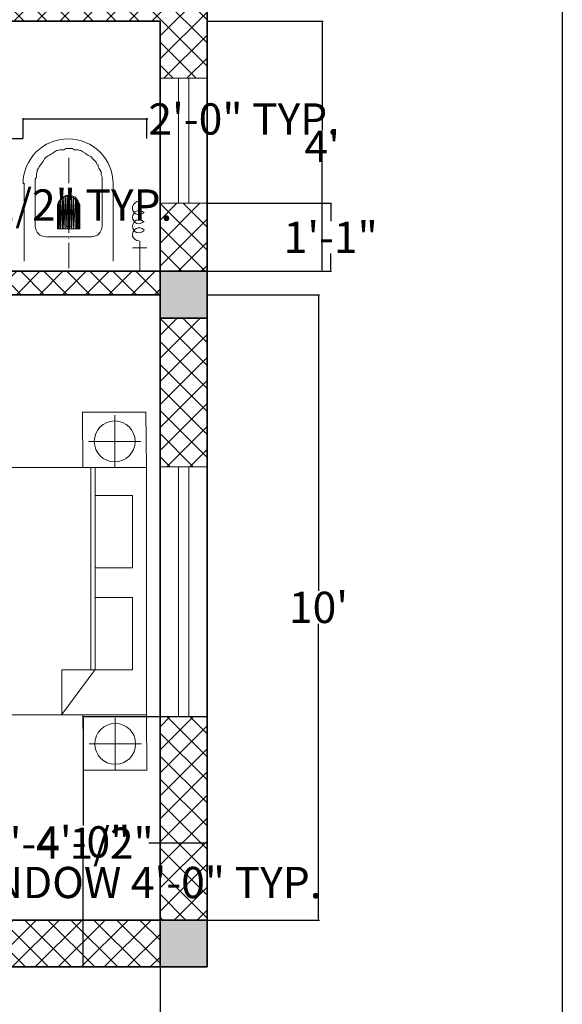
# Model space of a CAD drawing. Units: inches. Extents: x 958 to 1375, y 3152 to 3689.
# Tile 4 of 8: x 1271 to 1375, y 3251 to 3440. Entities that reach past the tile are written whole.
import ezdxf

# ---------------------------------------------------------------- set-up
doc = ezdxf.new("R2010")
doc.units = ezdxf.units.IN
doc.header["$MEASUREMENT"] = 0
for name, color, linetype, lineweight in [('A-ANNO-DIMS', 2, 'Continuous', 18), ('A-ANNO-TTLB', 7, 'Continuous', 25), ('A-COLS', 7, 'Continuous', 35), ('A-FLOR-FIXT', 8, 'Continuous', 18), ('A-FURN', 8, 'Continuous', 18), ('A-WALL', 7, 'Continuous', 35), ('windows', 140, 'Continuous', 18)]:
    doc.layers.add(name, color=color, linetype=linetype, lineweight=lineweight)
doc.layers.add('A-COLS-PATT', color=18, linetype='Continuous', lineweight=13, true_color=0x000000)
doc.layers.add('A-WALL-PATT', color=240, linetype='Continuous', lineweight=13, true_color=0xed1f24)
doc.styles.get("Standard").update_dxf_attribs({"font": 'arial.ttf'})
doc.dimstyles.get("Standard").update_dxf_attribs({"dimtxt": 6, "dimasz": 0.18, "dimexe": 0.18, "dimexo": 0.0625, "dimgap": 0.09, "dimtad": 0, "dimtih": 1, "dimtoh": 1, "dimdec": 1, "dimzin": 0, "dimdsep": 46, "dimlunit": 3, "dimtxsty": 'Standard', "dimcen": 0.09, "dimadec": 0, "dimazin": 0, "dimtfac": 1, "dimtdec": 1, "dimtofl": 0, "dimtmove": 0, "dimatfit": 3, "dimfxl": 1, "dimtolj": 1, "dimtzin": 0, "dimarcsym": 0})

# ---------------------------------------------------------------- blocks, each defined once
blk = doc.blocks.new('*D7')
at = {"layer": 'A-ANNO-DIMS', "color": 0, "lineweight": -2, "transparency": 16777216}
for p, q in [((1306.76, 3439.53), (1329, 3439.53)), ((1328.82, 3439.35), (1328.82, 3418.62)), ((1328.82, 3391.71), (1328.82, 3412.44)), ((1306.76, 3391.53), (1329, 3391.53))]:
    blk.add_line(p, q, dxfattribs=at)
at = {"layer": 'A-ANNO-DIMS', "color": 0, "transparency": 16777216}
for points in [[(1328.79, 3439.35), (1328.85, 3439.35), (1328.82, 3439.53)], [(1328.79, 3391.71), (1328.85, 3391.71), (1328.82, 3391.53)]]:
    blk.add_solid(points, dxfattribs=at)
at = {"layer": 'Defpoints', "color": 0, "transparency": 16777216}
for p in [(1306.7, 3439.53), (1306.7, 3391.53), (1328.82, 3391.53)]:
    blk.add_point(p, dxfattribs=at)
at = {"layer": 'A-ANNO-DIMS', "color": 0, "transparency": 16777216, "insert": (1328.82, 3415.53), "char_height": 6, "attachment_point": 5}
blk.add_mtext("\\A1;4'", dxfattribs=at)
blk = doc.blocks.new('*D8')
at = {"layer": 'A-ANNO-DIMS', "color": 0, "lineweight": -2, "transparency": 16777216}
for p, q in [((1306.76, 3387.03), (1328.29, 3387.03)), ((1328.11, 3386.85), (1328.11, 3330.19)), ((1328.11, 3267.21), (1328.11, 3323.88)), ((1306.76, 3267.03), (1328.29, 3267.03))]:
    blk.add_line(p, q, dxfattribs=at)
at = {"layer": 'A-ANNO-DIMS', "color": 0, "transparency": 16777216}
for points in [[(1328.08, 3386.85), (1328.14, 3386.85), (1328.11, 3387.03)], [(1328.08, 3267.21), (1328.14, 3267.21), (1328.11, 3267.03)]]:
    blk.add_solid(points, dxfattribs=at)
at = {"layer": 'Defpoints', "color": 0, "transparency": 16777216}
for p in [(1306.7, 3387.03), (1306.7, 3267.03), (1328.11, 3267.03)]:
    blk.add_point(p, dxfattribs=at)
at = {"layer": 'A-ANNO-DIMS', "color": 0, "transparency": 16777216, "insert": (1328.11, 3327.03), "char_height": 6, "attachment_point": 5}
blk.add_mtext("\\A1;10'", dxfattribs=at)
blk = doc.blocks.new('*D9')
at = {"layer": 'A-ANNO-DIMS', "color": 0, "lineweight": -2, "transparency": 16777216}
for p, q in [((1177.7, 3257.97), (1177.7, 3236.74)), ((1297.7, 3257.97), (1297.7, 3236.74)), ((1177.88, 3236.92), (1232.8, 3236.92)), ((1297.52, 3236.92), (1242.6, 3236.92))]:
    blk.add_line(p, q, dxfattribs=at)
at = {"layer": 'A-ANNO-DIMS', "color": 0, "transparency": 16777216}
for points in [[(1177.88, 3236.95), (1177.88, 3236.89), (1177.7, 3236.92)], [(1297.52, 3236.95), (1297.52, 3236.89), (1297.7, 3236.92)]]:
    blk.add_solid(points, dxfattribs=at)
at = {"layer": 'Defpoints', "color": 0, "transparency": 16777216}
for p in [(1177.7, 3258.03), (1297.7, 3258.03), (1177.7, 3236.92)]:
    blk.add_point(p, dxfattribs=at)
at = {"layer": 'A-ANNO-DIMS', "color": 0, "transparency": 16777216, "insert": (1237.7, 3236.92), "char_height": 6, "attachment_point": 5}
blk.add_mtext("\\A1;10'", dxfattribs=at)
blk = doc.blocks.new('BED-DOUBLE')
for p, q in [((5.6, 61.62), (5.6, 51.56)), ((63.65, 61.72), (63.65, 51.66)), ((68.68, 56.69), (58.62, 56.69)), ((10.63, 56.59), (0.57, 56.59)), ((49.39, 52.82), (10.63, 52.82)), ((49.44, 52), (10.63, 52)), ((49.39, 52.82), (58, 46.47)), ((49.44, 52.82), (49.44, 46.47)), ((49.44, 46.47), (58, 46.47)), ((58.05, 34.96), (10.63, 34.96)), ((4.36, 0), (4.36, 26.37)), ((4.36, 26.37), (10.65, 26.37)), ((58.05, 26.37), (67.59, 26.37)), ((67.59, 26.37), (67.59, 0)), ((67.59, 0), (4.36, 0))]:
    blk.add_line(p, q)
for points in [[(0, 50.39), (10.63, 50.5), (10.63, 62.68), (0, 62.58)], [(58.05, 62.68), (58.05, 11.37), (10.63, 11.37), (10.63, 62.68)], [(58.05, 50.5), (68.68, 50.6), (68.68, 62.78), (58.05, 62.68)], [(29.88, 59.98), (29.88, 52.82), (15.98, 52.82), (15.98, 59.98)], [(49.44, 59.98), (49.44, 52.82), (35.55, 52.82), (35.55, 59.98)]]:
    blk.add_lwpolyline(points, close=True)
for centre in [(5.6, 56.59), (63.65, 56.69)]:
    blk.add_circle(centre, 3.92)
for points, knots in [([(3.23, 25.84), (3.32, 25.96), (3.52, 26.2), (3.86, 25.96), (4.14, 25.78), (4.29, 25.89), (4.36, 25.94)], [0, 0, 0, 0, 0.400747, 0.791423, 1.067667, 1.29709, 1.29709, 1.29709, 1.29709]), ([(3.23, 25.06), (3.32, 25.18), (3.52, 25.42), (3.86, 25.18), (4.14, 25.01), (4.29, 25.11), (4.36, 25.16)], [0, 0, 0, 0, 0.400747, 0.791423, 1.067667, 1.29709, 1.29709, 1.29709, 1.29709]), ([(68.71, 25.84), (68.61, 25.96), (68.42, 26.2), (68.08, 25.96), (67.8, 25.78), (67.65, 25.89), (67.58, 25.94)], [0, 0, 0, 0, 0.400747, 0.791423, 1.067667, 1.29709, 1.29709, 1.29709, 1.29709]), ([(68.71, 25.06), (68.61, 25.18), (68.42, 25.42), (68.08, 25.18), (67.8, 25.01), (67.65, 25.11), (67.58, 25.16)], [0, 0, 0, 0, 0.400747, 0.791423, 1.067667, 1.29709, 1.29709, 1.29709, 1.29709]), ([(3.23, 24.24), (3.32, 24.36), (3.52, 24.6), (3.86, 24.36), (4.14, 24.19), (4.29, 24.3), (4.36, 24.34)], [0, 0, 0, 0, 0.400747, 0.791423, 1.067667, 1.29709, 1.29709, 1.29709, 1.29709]), ([(3.23, 23.51), (3.32, 23.63), (3.52, 23.87), (3.86, 23.63), (4.14, 23.46), (4.29, 23.57), (4.36, 23.62)], [0, 0, 0, 0, 0.400747, 0.791423, 1.067667, 1.29709, 1.29709, 1.29709, 1.29709]), ([(3.23, 22.63), (3.32, 22.75), (3.52, 22.99), (3.86, 22.75), (4.14, 22.58), (4.29, 22.69), (4.36, 22.73)], [0, 0, 0, 0, 0.400747, 0.791423, 1.067667, 1.29709, 1.29709, 1.29709, 1.29709]), ([(68.71, 24.24), (68.61, 24.36), (68.42, 24.6), (68.08, 24.36), (67.8, 24.19), (67.65, 24.3), (67.58, 24.34)], [0, 0, 0, 0, 0.400747, 0.791423, 1.067667, 1.29709, 1.29709, 1.29709, 1.29709]), ([(68.71, 23.51), (68.61, 23.63), (68.42, 23.87), (68.08, 23.63), (67.8, 23.46), (67.65, 23.57), (67.58, 23.62)], [0, 0, 0, 0, 0.400747, 0.791423, 1.067667, 1.29709, 1.29709, 1.29709, 1.29709]), ([(68.71, 22.63), (68.61, 22.75), (68.42, 22.99), (68.08, 22.75), (67.8, 22.58), (67.65, 22.69), (67.58, 22.73)], [0, 0, 0, 0, 0.400747, 0.791423, 1.067667, 1.29709, 1.29709, 1.29709, 1.29709]), ([(3.23, 21.88), (3.32, 22), (3.52, 22.24), (3.86, 22), (4.14, 21.83), (4.29, 21.93), (4.36, 21.98)], [0, 0, 0, 0, 0.400747, 0.791423, 1.067667, 1.29709, 1.29709, 1.29709, 1.29709]), ([(3.23, 21.15), (3.32, 21.27), (3.52, 21.51), (3.86, 21.27), (4.14, 21.1), (4.29, 21.21), (4.36, 21.25)], [0, 0, 0, 0, 0.400747, 0.791423, 1.067667, 1.29709, 1.29709, 1.29709, 1.29709]), ([(68.71, 21.88), (68.61, 22), (68.42, 22.24), (68.08, 22), (67.8, 21.83), (67.65, 21.93), (67.58, 21.98)], [0, 0, 0, 0, 0.400747, 0.791423, 1.067667, 1.29709, 1.29709, 1.29709, 1.29709]), ([(68.71, 21.15), (68.61, 21.27), (68.42, 21.51), (68.08, 21.27), (67.8, 21.1), (67.65, 21.21), (67.58, 21.25)], [0, 0, 0, 0, 0.400747, 0.791423, 1.067667, 1.29709, 1.29709, 1.29709, 1.29709]), ([(3.23, 20.27), (3.32, 20.39), (3.52, 20.63), (3.86, 20.39), (4.14, 20.22), (4.29, 20.32), (4.36, 20.37)], [0, 0, 0, 0, 0.400747, 0.791423, 1.067667, 1.29709, 1.29709, 1.29709, 1.29709]), ([(3.23, 19.23), (3.32, 19.35), (3.52, 19.59), (3.86, 19.35), (4.14, 19.18), (4.29, 19.29), (4.36, 19.33)], [0, 0, 0, 0, 0.400747, 0.791423, 1.067667, 1.29709, 1.29709, 1.29709, 1.29709]), ([(68.71, 20.27), (68.61, 20.39), (68.42, 20.63), (68.08, 20.39), (67.8, 20.22), (67.65, 20.32), (67.58, 20.37)], [0, 0, 0, 0, 0.400747, 0.791423, 1.067667, 1.29709, 1.29709, 1.29709, 1.29709]), ([(68.71, 19.23), (68.61, 19.35), (68.42, 19.59), (68.08, 19.35), (67.8, 19.18), (67.65, 19.29), (67.58, 19.33)], [0, 0, 0, 0, 0.400747, 0.791423, 1.067667, 1.29709, 1.29709, 1.29709, 1.29709]), ([(3.23, 18.35), (3.32, 18.47), (3.52, 18.71), (3.86, 18.47), (4.14, 18.3), (4.29, 18.4), (4.36, 18.45)], [0, 0, 0, 0, 0.400747, 0.791423, 1.067667, 1.29709, 1.29709, 1.29709, 1.29709]), ([(3.23, 17.53), (3.32, 17.65), (3.52, 17.89), (3.86, 17.65), (4.14, 17.48), (4.29, 17.59), (4.36, 17.64)], [0, 0, 0, 0, 0.400747, 0.791423, 1.067667, 1.29709, 1.29709, 1.29709, 1.29709]), ([(3.23, 16.76), (3.32, 16.88), (3.52, 17.12), (3.86, 16.88), (4.14, 16.71), (4.29, 16.81), (4.36, 16.86)], [0, 0, 0, 0, 0.400747, 0.791423, 1.067667, 1.29709, 1.29709, 1.29709, 1.29709]), ([(68.71, 18.35), (68.61, 18.47), (68.42, 18.71), (68.08, 18.47), (67.8, 18.3), (67.65, 18.4), (67.58, 18.45)], [0, 0, 0, 0, 0.400747, 0.791423, 1.067667, 1.29709, 1.29709, 1.29709, 1.29709]), ([(68.71, 17.53), (68.61, 17.65), (68.42, 17.89), (68.08, 17.65), (67.8, 17.48), (67.65, 17.59), (67.58, 17.64)], [0, 0, 0, 0, 0.400747, 0.791423, 1.067667, 1.29709, 1.29709, 1.29709, 1.29709]), ([(68.71, 16.76), (68.61, 16.88), (68.42, 17.12), (68.08, 16.88), (67.8, 16.71), (67.65, 16.81), (67.58, 16.86)], [0, 0, 0, 0, 0.400747, 0.791423, 1.067667, 1.29709, 1.29709, 1.29709, 1.29709]), ([(3.23, 15.94), (3.32, 16.06), (3.52, 16.3), (3.86, 16.06), (4.14, 15.89), (4.29, 16), (4.36, 16.04)], [0, 0, 0, 0, 0.400747, 0.791423, 1.067667, 1.29709, 1.29709, 1.29709, 1.29709]), ([(3.23, 15.21), (3.32, 15.33), (3.52, 15.57), (3.86, 15.33), (4.14, 15.16), (4.29, 15.27), (4.36, 15.32)], [0, 0, 0, 0, 0.400747, 0.791423, 1.067667, 1.29709, 1.29709, 1.29709, 1.29709]), ([(68.71, 15.94), (68.61, 16.06), (68.42, 16.3), (68.08, 16.06), (67.8, 15.89), (67.65, 16), (67.58, 16.04)], [0, 0, 0, 0, 0.400747, 0.791423, 1.067667, 1.29709, 1.29709, 1.29709, 1.29709]), ([(68.71, 15.21), (68.61, 15.33), (68.42, 15.57), (68.08, 15.33), (67.8, 15.16), (67.65, 15.27), (67.58, 15.32)], [0, 0, 0, 0, 0.400747, 0.791423, 1.067667, 1.29709, 1.29709, 1.29709, 1.29709]), ([(3.23, 14.33), (3.32, 14.45), (3.52, 14.69), (3.86, 14.45), (4.14, 14.28), (4.29, 14.39), (4.36, 14.43)], [0, 0, 0, 0, 0.400747, 0.791423, 1.067667, 1.29709, 1.29709, 1.29709, 1.29709]), ([(3.23, 13.58), (3.32, 13.7), (3.52, 13.94), (3.86, 13.7), (4.14, 13.53), (4.29, 13.63), (4.36, 13.68)], [0, 0, 0, 0, 0.400747, 0.791423, 1.067667, 1.29709, 1.29709, 1.29709, 1.29709]), ([(68.71, 14.33), (68.61, 14.45), (68.42, 14.69), (68.08, 14.45), (67.8, 14.28), (67.65, 14.39), (67.58, 14.43)], [0, 0, 0, 0, 0.400747, 0.791423, 1.067667, 1.29709, 1.29709, 1.29709, 1.29709]), ([(68.71, 13.58), (68.61, 13.7), (68.42, 13.94), (68.08, 13.7), (67.8, 13.53), (67.65, 13.63), (67.58, 13.68)], [0, 0, 0, 0, 0.400747, 0.791423, 1.067667, 1.29709, 1.29709, 1.29709, 1.29709]), ([(3.23, 12.85), (3.32, 12.97), (3.52, 13.21), (3.86, 12.97), (4.14, 12.8), (4.29, 12.9), (4.36, 12.95)], [0, 0, 0, 0, 0.400747, 0.791423, 1.067667, 1.29709, 1.29709, 1.29709, 1.29709]), ([(3.23, 11.97), (3.32, 12.09), (3.52, 12.33), (3.86, 12.09), (4.14, 11.92), (4.29, 12.02), (4.36, 12.07)], [0, 0, 0, 0, 0.400747, 0.791423, 1.067667, 1.29709, 1.29709, 1.29709, 1.29709]), ([(68.71, 12.85), (68.61, 12.97), (68.42, 13.21), (68.08, 12.97), (67.8, 12.8), (67.65, 12.9), (67.58, 12.95)], [0, 0, 0, 0, 0.400747, 0.791423, 1.067667, 1.29709, 1.29709, 1.29709, 1.29709]), ([(68.71, 11.97), (68.61, 12.09), (68.42, 12.33), (68.08, 12.09), (67.8, 11.92), (67.65, 12.02), (67.58, 12.07)], [0, 0, 0, 0, 0.400747, 0.791423, 1.067667, 1.29709, 1.29709, 1.29709, 1.29709]), ([(3.23, 10.93), (3.32, 11.05), (3.52, 11.29), (3.86, 11.05), (4.14, 10.88), (4.29, 10.99), (4.36, 11.03)], [0, 0, 0, 0, 0.400747, 0.791423, 1.067667, 1.29709, 1.29709, 1.29709, 1.29709]), ([(3.23, 10.05), (3.32, 10.17), (3.52, 10.41), (3.86, 10.17), (4.14, 10), (4.29, 10.1), (4.36, 10.15)], [0, 0, 0, 0, 0.400747, 0.791423, 1.067667, 1.29709, 1.29709, 1.29709, 1.29709]), ([(3.23, 9.23), (3.32, 9.35), (3.52, 9.59), (3.86, 9.35), (4.14, 9.18), (4.29, 9.29), (4.36, 9.34)], [0, 0, 0, 0, 0.400747, 0.791423, 1.067667, 1.29709, 1.29709, 1.29709, 1.29709]), ([(68.71, 10.93), (68.61, 11.05), (68.42, 11.29), (68.08, 11.05), (67.8, 10.88), (67.65, 10.99), (67.58, 11.03)], [0, 0, 0, 0, 0.400747, 0.791423, 1.067667, 1.29709, 1.29709, 1.29709, 1.29709]), ([(68.71, 10.05), (68.61, 10.17), (68.42, 10.41), (68.08, 10.17), (67.8, 10), (67.65, 10.1), (67.58, 10.15)], [0, 0, 0, 0, 0.400747, 0.791423, 1.067667, 1.29709, 1.29709, 1.29709, 1.29709]), ([(68.71, 9.23), (68.61, 9.35), (68.42, 9.59), (68.08, 9.35), (67.8, 9.18), (67.65, 9.29), (67.58, 9.34)], [0, 0, 0, 0, 0.400747, 0.791423, 1.067667, 1.29709, 1.29709, 1.29709, 1.29709]), ([(3.23, 8.54), (3.32, 8.66), (3.52, 8.9), (3.86, 8.66), (4.14, 8.49), (4.29, 8.6), (4.36, 8.65)], [0, 0, 0, 0, 0.400747, 0.791423, 1.067667, 1.29709, 1.29709, 1.29709, 1.29709]), ([(3.23, 7.73), (3.32, 7.85), (3.52, 8.09), (3.86, 7.85), (4.14, 7.68), (4.29, 7.78), (4.36, 7.83)], [0, 0, 0, 0, 0.400747, 0.791423, 1.067667, 1.29709, 1.29709, 1.29709, 1.29709]), ([(68.71, 8.54), (68.61, 8.66), (68.42, 8.9), (68.08, 8.66), (67.8, 8.49), (67.65, 8.6), (67.58, 8.65)], [0, 0, 0, 0, 0.400747, 0.791423, 1.067667, 1.29709, 1.29709, 1.29709, 1.29709]), ([(68.71, 7.73), (68.61, 7.85), (68.42, 8.09), (68.08, 7.85), (67.8, 7.68), (67.65, 7.78), (67.58, 7.83)], [0, 0, 0, 0, 0.400747, 0.791423, 1.067667, 1.29709, 1.29709, 1.29709, 1.29709]), ([(3.23, 7), (3.32, 7.12), (3.52, 7.36), (3.86, 7.12), (4.14, 6.95), (4.29, 7.05), (4.36, 7.1)], [0, 0, 0, 0, 0.400747, 0.791423, 1.067667, 1.29709, 1.29709, 1.29709, 1.29709]), ([(3.23, 6.12), (3.32, 6.24), (3.52, 6.48), (3.86, 6.24), (4.14, 6.07), (4.29, 6.17), (4.36, 6.22)], [0, 0, 0, 0, 0.400747, 0.791423, 1.067667, 1.29709, 1.29709, 1.29709, 1.29709]), ([(68.71, 7), (68.61, 7.12), (68.42, 7.36), (68.08, 7.12), (67.8, 6.95), (67.65, 7.05), (67.58, 7.1)], [0, 0, 0, 0, 0.400747, 0.791423, 1.067667, 1.29709, 1.29709, 1.29709, 1.29709]), ([(68.71, 6.12), (68.61, 6.24), (68.42, 6.48), (68.08, 6.24), (67.8, 6.07), (67.65, 6.17), (67.58, 6.22)], [0, 0, 0, 0, 0.400747, 0.791423, 1.067667, 1.29709, 1.29709, 1.29709, 1.29709]), ([(3.23, 5.37), (3.32, 5.49), (3.52, 5.73), (3.86, 5.49), (4.14, 5.31), (4.29, 5.42), (4.36, 5.47)], [0, 0, 0, 0, 0.400747, 0.791423, 1.067667, 1.29709, 1.29709, 1.29709, 1.29709]), ([(3.23, 4.64), (3.32, 4.76), (3.52, 5), (3.86, 4.76), (4.14, 4.59), (4.29, 4.69), (4.36, 4.74)], [0, 0, 0, 0, 0.400747, 0.791423, 1.067667, 1.29709, 1.29709, 1.29709, 1.29709]), ([(3.23, 3.75), (3.32, 3.88), (3.52, 4.12), (3.86, 3.88), (4.14, 3.7), (4.29, 3.81), (4.36, 3.86)], [0, 0, 0, 0, 0.400747, 0.791423, 1.067667, 1.29709, 1.29709, 1.29709, 1.29709]), ([(68.71, 5.37), (68.61, 5.49), (68.42, 5.73), (68.08, 5.49), (67.8, 5.31), (67.65, 5.42), (67.58, 5.47)], [0, 0, 0, 0, 0.400747, 0.791423, 1.067667, 1.29709, 1.29709, 1.29709, 1.29709]), ([(68.71, 4.64), (68.61, 4.76), (68.42, 5), (68.08, 4.76), (67.8, 4.59), (67.66, 4.69), (67.59, 4.73)], [0, 0, 0, 0, 0.400747, 0.791423, 1.067667, 1.283686, 1.283686, 1.283686, 1.283686]), ([(68.71, 3.75), (68.61, 3.88), (68.42, 4.12), (68.08, 3.88), (67.8, 3.7), (67.66, 3.81), (67.59, 3.85)], [0, 0, 0, 0, 0.400747, 0.791423, 1.067667, 1.283686, 1.283686, 1.283686, 1.283686]), ([(3.23, 3.33), (3.32, 3.45), (3.52, 3.7), (3.86, 3.45), (4.14, 3.27), (4.29, 3.38), (4.36, 3.43)], [0, 0, 0, 0, 0.407265, 0.802015, 1.07826, 1.307683, 1.307683, 1.307683, 1.307683]), ([(3.23, 2.76), (3.32, 2.88), (3.52, 3.12), (3.86, 2.88), (4.14, 2.71), (4.29, 2.81), (4.36, 2.86)], [0, 0, 0, 0, 0.400747, 0.791423, 1.067667, 1.29709, 1.29709, 1.29709, 1.29709]), ([(3.23, 2.19), (3.32, 2.31), (3.52, 2.55), (3.86, 2.31), (4.14, 2.13), (4.29, 2.24), (4.36, 2.29)], [0, 0, 0, 0, 0.400747, 0.791423, 1.067667, 1.29709, 1.29709, 1.29709, 1.29709]), ([(3.23, 1.88), (3.32, 2), (3.52, 2.24), (3.86, 2), (4.14, 1.82), (4.29, 1.93), (4.36, 1.98)], [0, 0, 0, 0, 0.400747, 0.791423, 1.067667, 1.29709, 1.29709, 1.29709, 1.29709]), ([(68.71, 3.33), (68.61, 3.45), (68.42, 3.69), (68.08, 3.45), (67.8, 3.28), (67.66, 3.38), (67.59, 3.42)], [0, 0, 0, 0, 0.402903, 0.794912, 1.071156, 1.287177, 1.287177, 1.287177, 1.287177]), ([(68.71, 2.73), (68.61, 2.85), (68.42, 3.09), (68.08, 2.85), (67.8, 2.68), (67.66, 2.78), (67.59, 2.83)], [0, 0, 0, 0, 0.400747, 0.791423, 1.067667, 1.283686, 1.283686, 1.283686, 1.283686]), ([(68.71, 2.16), (68.61, 2.28), (68.42, 2.52), (68.08, 2.28), (67.8, 2.11), (67.66, 2.21), (67.59, 2.25)], [0, 0, 0, 0, 0.400747, 0.791423, 1.067667, 1.283686, 1.283686, 1.283686, 1.283686]), ([(68.71, 1.85), (68.61, 1.97), (68.42, 2.21), (68.08, 1.97), (67.8, 1.8), (67.66, 1.9), (67.59, 1.94)], [0, 0, 0, 0, 0.400747, 0.791423, 1.067667, 1.283686, 1.283686, 1.283686, 1.283686]), ([(3.23, 1.46), (3.32, 1.58), (3.52, 1.82), (3.86, 1.58), (4.14, 1.41), (4.29, 1.51), (4.36, 1.56)], [0, 0, 0, 0, 0.400747, 0.791423, 1.067667, 1.29709, 1.29709, 1.29709, 1.29709]), ([(3.23, 1.06), (3.32, 1.18), (3.52, 1.42), (3.86, 1.18), (4.14, 1.01), (4.29, 1.11), (4.36, 1.16)], [0, 0, 0, 0, 0.400747, 0.791423, 1.067667, 1.29709, 1.29709, 1.29709, 1.29709]), ([(3.23, 0.57), (3.32, 0.7), (3.52, 0.94), (3.86, 0.7), (4.14, 0.52), (4.29, 0.63), (4.36, 0.68)], [0, 0, 0, 0, 0.400747, 0.791423, 1.067667, 1.29709, 1.29709, 1.29709, 1.29709]), ([(3.23, 0.07), (3.32, 0.19), (3.52, 0.43), (3.86, 0.19), (4.14, 0.02), (4.29, 0.13), (4.36, 0.18)], [0, 0, 0, 0, 0.400747, 0.791423, 1.067667, 1.29709, 1.29709, 1.29709, 1.29709]), ([(68.71, 1.43), (68.61, 1.55), (68.42, 1.79), (68.08, 1.55), (67.8, 1.38), (67.65, 1.48), (67.58, 1.53)], [0, 0, 0, 0, 0.400747, 0.791423, 1.067667, 1.29709, 1.29709, 1.29709, 1.29709]), ([(68.71, 1.03), (68.61, 1.15), (68.42, 1.39), (68.08, 1.15), (67.8, 0.98), (67.65, 1.09), (67.58, 1.13)], [0, 0, 0, 0, 0.400747, 0.791423, 1.067667, 1.29709, 1.29709, 1.29709, 1.29709]), ([(68.71, 0.55), (68.61, 0.67), (68.42, 0.91), (68.08, 0.67), (67.8, 0.5), (67.65, 0.6), (67.58, 0.65)], [0, 0, 0, 0, 0.400747, 0.791423, 1.067667, 1.29709, 1.29709, 1.29709, 1.29709]), ([(68.71, 0.07), (68.61, 0.19), (68.42, 0.43), (68.08, 0.19), (67.8, 0.02), (67.65, 0.13), (67.58, 0.18)], [0, 0, 0, 0, 0.400747, 0.791423, 1.067667, 1.29709, 1.29709, 1.29709, 1.29709])]:
    blk.add_open_spline(points, degree=3, knots=knots)
blk = doc.blocks.new('WC-PLAN')
h = blk.add_hatch(color=256)
h.paths.add_polyline_path([(7.05, 8.12), (7.05, 13.58), (6.83, 8.12)])
h.paths.add_polyline_path([(7.05, 13.58), (6.83, 8.12), (6.83, 13.2)])
h = blk.add_hatch(color=256)
h.paths.add_polyline_path([(7.21, 8.12), (7.21, 13.81), (7.05, 8.12)])
h.paths.add_polyline_path([(7.21, 13.81), (7.05, 8.12), (7.05, 13.58)])
h = blk.add_hatch(color=256)
h.paths.add_polyline_path([(7.59, 8.12), (7.59, 14.19), (7.21, 8.12)])
h.paths.add_polyline_path([(7.59, 14.19), (7.21, 8.12), (7.21, 13.81)])
h = blk.add_hatch(color=256)
h.paths.add_polyline_path([(7.81, 8.12), (7.81, 14.34), (7.59, 8.12)])
h.paths.add_polyline_path([(7.81, 14.34), (7.59, 8.12), (7.59, 14.19)])
h = blk.add_hatch(color=256)
h.paths.add_polyline_path([(8.19, 8.12), (8.19, 14.56), (7.81, 8.12)])
h.paths.add_polyline_path([(8.19, 14.56), (7.81, 8.12), (7.81, 14.34)])
h = blk.add_hatch(color=256)
h.paths.add_polyline_path([(8.57, 8.12), (8.57, 14.56), (8.19, 8.12)])
h.paths.add_polyline_path([(8.57, 14.56), (8.19, 8.12), (8.19, 14.56)])
h = blk.add_hatch(color=256)
h.paths.add_polyline_path([(8.95, 8.12), (8.95, 14.56), (8.57, 8.12)])
h.paths.add_polyline_path([(8.95, 14.56), (8.57, 8.12), (8.57, 14.56)])
h = blk.add_hatch(color=256)
h.paths.add_polyline_path([(9.33, 8.12), (9.33, 14.56), (8.95, 8.12)])
h.paths.add_polyline_path([(9.33, 14.56), (8.95, 8.12), (8.95, 14.56)])
h = blk.add_hatch(color=256)
h.paths.add_polyline_path([(9.71, 8.12), (9.71, 14.34), (9.33, 8.12)])
h.paths.add_polyline_path([(9.71, 14.34), (9.33, 8.12), (9.33, 14.56)])
h = blk.add_hatch(color=256)
h.paths.add_polyline_path([(10.16, 8.12), (10.16, 14.19), (9.71, 8.12)])
h.paths.add_polyline_path([(10.16, 14.19), (9.71, 8.12), (9.71, 14.34)])
h = blk.add_hatch(color=256)
h.paths.add_polyline_path([(10.32, 8.12), (10.32, 13.81), (10.16, 8.12)])
h.paths.add_polyline_path([(10.32, 13.81), (10.16, 8.12), (10.16, 14.19)])
h = blk.add_hatch(color=256)
h.paths.add_polyline_path([(10.54, 8.12), (10.54, 13.58), (10.32, 8.12)])
h.paths.add_polyline_path([(10.54, 13.58), (10.32, 8.12), (10.32, 13.81)])
h = blk.add_hatch(color=256)
h.paths.add_polyline_path([(10.7, 8.12), (10.7, 13.2), (10.54, 8.12)])
h.paths.add_polyline_path([(10.7, 13.2), (10.54, 8.12), (10.54, 13.58)])
h = blk.add_hatch(color=256)
h.paths.add_polyline_path([(6.83, 8.12), (6.83, 13.2), (6.6, 8.12)])
h.paths.add_polyline_path([(6.83, 13.2), (6.6, 8.12), (6.6, 12.82)])
h.paths.add_polyline_path([(6.6, 8.12), (6.6, 12.82), (6.6, 12.44)])
h = blk.add_hatch(color=256)
h.paths.add_polyline_path([(10.92, 8.12), (10.92, 12.82), (10.7, 8.12)])
h.paths.add_polyline_path([(10.92, 12.82), (10.7, 8.12), (10.7, 13.2)])
for points in [[(2.35, 15.93), (2.35, 16.69), (2.35, 17.3), (2.35, 17.67), (2.58, 18.05), (2.58, 18.43), (2.58, 18.66), (2.73, 19.04), (2.73, 19.42), (2.96, 19.8), (3.11, 20.03), (3.34, 20.41), (3.49, 20.56), (3.72, 20.94), (3.94, 21.16), (4.1, 21.54), (4.32, 21.77), (4.48, 21.92), (4.85, 22.15), (5.08, 22.3), (5.46, 22.53), (5.69, 22.68), (6.07, 22.91), (6.45, 23.14), (6.6, 23.14), (7.05, 23.29), (7.43, 23.29), (7.81, 23.29), (8.19, 23.52), (8.8, 23.52), (9.56, 23.52), (9.71, 23.29), (10.16, 23.29), (10.54, 23.29), (10.92, 23.14), (11.07, 23.14), (11.45, 22.91), (11.91, 22.68), (12.06, 22.53), (12.44, 22.3), (12.67, 22.15), (13.05, 21.92), (13.2, 21.77), (13.43, 21.54), (13.81, 21.16), (14.03, 20.94), (14.18, 20.56), (14.41, 20.41), (14.41, 20.03), (14.56, 19.8), (14.79, 19.42), (15.02, 19.04), (15.02, 18.66), (15.02, 18.43), (15.17, 18.05), (15.17, 17.67), (15.17, 17.3), (15.17, 16.69), (15.17, 15.93)], [(8.8, 16.92), (8.8, 21.77), (8.8, 21.77)], [(0.23, 1.9), (0.23, 16.92), (0.23, 16.92)], [(2.35, 8.72), (2.35, 15.93), (2.35, 15.93)], [(15.17, 8.72), (15.17, 15.93), (15.17, 15.93)], [(17.3, 1.9), (17.3, 16.92), (17.3, 16.92)], [(8.8, 7.36), (8.8, 14.94), (8.8, 14.94)], [(6.6, 8.12), (6.6, 12.44), (6.6, 12.44)], [(10.92, 8.12), (10.92, 12.44), (10.92, 12.44)], [(6.6, 8.12), (10.92, 8.12), (10.92, 8.12)], [(8.34, 8.57), (8.57, 8.57), (8.8, 8.57)], [(8.34, 8.57), (8.34, 8.5), (8.34, 8.5)], [(8.8, 8.57), (8.72, 8.5), (8.72, 8.5)], [(8.8, 8.57), (8.95, 8.57), (9.18, 8.57)], [(9.18, 8.57), (9.18, 8.5), (9.18, 8.5)], [(4.48, 6.6), (13.2, 6.6), (13.2, 6.6)], [(8.8, 6.37), (8.72, 6.37), (8.72, 6.37)], [(22.4, 0), (22.4, 5.84), (22.4, 5.84)], [(8.8, 0.61), (8.8, 5.46), (8.8, 5.46)], [(21.03, 4.48), (23.77, 4.48), (23.77, 4.48)]]:
    blk.add_lwpolyline(points)
for points in [[(7.05, 8.12), (7.05, 13.58), (6.83, 8.12)], [(7.05, 13.58), (6.83, 8.12), (6.83, 13.2)], [(7.21, 8.12), (7.21, 13.81), (7.05, 8.12)], [(7.21, 13.81), (7.05, 8.12), (7.05, 13.58)], [(7.59, 8.12), (7.59, 14.19), (7.21, 8.12)], [(7.59, 14.19), (7.21, 8.12), (7.21, 13.81)], [(7.81, 8.12), (7.81, 14.34), (7.59, 8.12)], [(7.81, 14.34), (7.59, 8.12), (7.59, 14.19)], [(8.19, 8.12), (8.19, 14.56), (7.81, 8.12)], [(8.19, 14.56), (7.81, 8.12), (7.81, 14.34)], [(8.57, 8.12), (8.57, 14.56), (8.19, 8.12)], [(8.57, 14.56), (8.19, 8.12), (8.19, 14.56)], [(8.95, 8.12), (8.95, 14.56), (8.57, 8.12)], [(8.95, 14.56), (8.57, 8.12), (8.57, 14.56)], [(9.33, 8.12), (9.33, 14.56), (8.95, 8.12)], [(9.33, 14.56), (8.95, 8.12), (8.95, 14.56)], [(9.71, 14.34), (9.33, 8.12), (9.33, 14.56)], [(9.71, 8.12), (9.71, 14.34), (9.33, 8.12)], [(10.16, 14.19), (9.71, 8.12), (9.71, 14.34)], [(10.16, 8.12), (10.16, 14.19), (9.71, 8.12)], [(10.32, 13.81), (10.16, 8.12), (10.16, 14.19)], [(10.32, 8.12), (10.32, 13.81), (10.16, 8.12)], [(10.54, 13.58), (10.32, 8.12), (10.32, 13.81)], [(10.54, 8.12), (10.54, 13.58), (10.32, 8.12)], [(10.7, 13.2), (10.54, 8.12), (10.54, 13.58)], [(6.83, 8.12), (6.83, 13.2), (6.6, 8.12)], [(6.83, 13.2), (6.6, 8.12), (6.6, 12.82)], [(6.6, 8.12), (6.6, 12.82), (6.6, 12.44)], [(6.6, 12.82), (6.6, 8.12), (6.6, 8.12)], [(10.7, 8.12), (10.7, 13.2), (10.54, 8.12)], [(10.92, 12.82), (10.7, 8.12), (10.7, 13.2)], [(10.92, 8.12), (10.92, 12.82), (10.7, 8.12)], [(10.92, 12.44), (10.92, 8.12), (10.92, 12.82)], [(10.92, 8.12), (10.92, 12.44)]]:
    blk.add_lwpolyline(points, close=True)
for points, knots in [([(17.3, 16.76), (17.3, 21.54), (13.43, 25.41), (8.65, 25.41), (8.65, 25.41), (3.87, 25.41), (0, 21.54), (0, 16.76)], [0, 0, 0, 0, 0.125, 0.125, 0.125, 0.125001, 1, 1, 1, 1]), ([(10.7, 12.29), (10.7, 13.43), (9.79, 14.34), (8.65, 14.34), (8.65, 14.34), (7.51, 14.34), (6.6, 13.43), (6.6, 12.29)], [0, 0, 0, 0, 0.125, 0.125, 0.125, 0.125001, 1, 1, 1, 1]), ([(22.25, 13.43), (21.72, 13.43), (21.19, 12.97), (21.03, 12.44), (21.03, 12.44), (20.88, 11.91), (21.19, 11.3), (21.64, 11), (21.64, 11), (22.17, 10.77), (22.78, 10.85), (23.16, 11.23)], [0, 0, 0, 0, 0.083333, 0.083333, 0.083333, 0.083334, 0.166667, 0.166667, 0.166667, 0.166668, 1, 1, 1, 1]), ([(23.23, 11.23), (22.86, 11.61), (22.32, 11.76), (21.79, 11.53), (21.79, 11.53), (21.34, 11.38), (21.03, 10.92), (21.03, 10.39), (21.03, 10.39), (21.03, 9.86), (21.34, 9.41), (21.79, 9.18), (21.79, 9.18), (22.32, 9.03), (22.86, 9.18), (23.23, 9.56)], [0, 0, 0, 0, 0.0625, 0.0625, 0.0625, 0.062501, 0.125, 0.125, 0.125, 0.125001, 0.1875, 0.1875, 0.1875, 0.187501, 1, 1, 1, 1]), ([(23.16, 9.48), (22.86, 9.86), (22.25, 10.01), (21.79, 9.79), (21.79, 9.79), (21.34, 9.63), (21.03, 9.1), (21.03, 8.65), (21.03, 8.65), (21.03, 8.12), (21.34, 7.66), (21.79, 7.43), (21.79, 7.43), (22.32, 7.28), (22.86, 7.43), (23.23, 7.81)], [0, 0, 0, 0, 0.0625, 0.0625, 0.0625, 0.062501, 0.125, 0.125, 0.125, 0.125001, 0.1875, 0.1875, 0.1875, 0.187501, 1, 1, 1, 1]), ([(23.23, 7.97), (22.86, 8.34), (22.17, 8.5), (21.72, 8.19), (21.72, 8.19), (21.19, 7.89), (20.88, 7.36), (21.03, 6.75), (21.03, 6.75), (21.19, 6.22), (21.72, 5.84), (22.25, 5.84)], [0, 0, 0, 0, 0.083333, 0.083333, 0.083333, 0.083334, 0.166667, 0.166667, 0.166667, 0.166668, 1, 1, 1, 1])]:
    blk.add_open_spline(points, degree=3, knots=knots)
for points in [[(2.35, 8.65), (2.35, 7.51), (3.26, 6.6), (4.4, 6.6)], [(13.12, 6.6), (14.26, 6.6), (15.17, 7.51), (15.17, 8.65)]]:
    blk.add_open_spline(points, degree=3)
blk = doc.blocks.new('WIN-48')
for p, q in [((48, 9), (0, 9)), ((48, 5.5), (0, 5.5)), ((0, 3.5), (48, 3.5)), ((0, 0), (48, 0))]:
    blk.add_line(p, q)
blk = doc.blocks.new('VENT-24')
for p, q in [((0, 0), (0, 24)), ((3.5, 0), (3.5, 24)), ((5.5, 24), (5.5, 0)), ((9, 24), (9, 0))]:
    blk.add_line(p, q)
blk = doc.blocks.new('*D22')
at = {"layer": 'A-ANNO-DIMS', "color": 0, "lineweight": -2, "transparency": 16777216}
for p, q in [((1206.05, 3267.1), (1206.05, 3274.41)), ((1206.23, 3274.23), (1253.87, 3274.23)), ((1254.05, 3267.1), (1254.05, 3274.41)), ((1254.05, 3274.23), (1254.23, 3274.23))]:
    blk.add_line(p, q, dxfattribs=at)
at = {"layer": 'A-ANNO-DIMS', "color": 0, "transparency": 16777216}
for points in [[(1206.23, 3274.26), (1206.23, 3274.2), (1206.05, 3274.23)], [(1253.87, 3274.26), (1253.87, 3274.2), (1254.05, 3274.23)]]:
    blk.add_solid(points, dxfattribs=at)
at = {"layer": 'Defpoints', "color": 0, "transparency": 16777216}
for p in [(1254.05, 3274.23), (1206.05, 3267.03), (1254.05, 3267.03)]:
    blk.add_point(p, dxfattribs=at)
at = {"layer": 'A-ANNO-DIMS', "color": 0, "transparency": 16777216, "insert": (1292.28, 3274.23), "char_height": 6, "attachment_point": 5}
blk.add_mtext('\\A1;WINDOW 4\'-0" TYP.', dxfattribs=at)
blk = doc.blocks.new('*D28')
at = {"layer": 'A-ANNO-DIMS', "color": 0, "lineweight": -2, "transparency": 16777216}
for p, q in [((1271.31, 3416.95), (1267.38, 3416.95)), ((1267.56, 3416.77), (1267.56, 3407.43)), ((1267.56, 3391.72), (1267.56, 3401.05)), ((1271.31, 3391.54), (1267.38, 3391.54))]:
    blk.add_line(p, q, dxfattribs=at)
at = {"layer": 'A-ANNO-DIMS', "color": 0, "transparency": 16777216}
for points in [[(1267.53, 3416.77), (1267.59, 3416.77), (1267.56, 3416.95)], [(1267.53, 3391.72), (1267.59, 3391.72), (1267.56, 3391.54)]]:
    blk.add_solid(points, dxfattribs=at)
at = {"layer": 'Defpoints', "color": 0, "transparency": 16777216}
for p in [(1267.56, 3416.95), (1271.38, 3416.95), (1271.38, 3391.54)]:
    blk.add_point(p, dxfattribs=at)
at = {"layer": 'A-ANNO-DIMS', "color": 0, "transparency": 16777216, "insert": (1267.56, 3404.24), "char_height": 6, "attachment_point": 5}
blk.add_mtext('\\A1;WC 2\'-1 1/2" TYP.', dxfattribs=at)
blk = doc.blocks.new('*D29')
at = {"layer": 'A-ANNO-DIMS', "color": 0, "lineweight": -2, "transparency": 16777216}
for p, q in [((1271.38, 3417.01), (1271.38, 3420.94)), ((1271.56, 3420.76), (1294.96, 3420.76)), ((1295.14, 3417.01), (1295.14, 3420.94)), ((1295.14, 3420.76), (1295.32, 3420.76))]:
    blk.add_line(p, q, dxfattribs=at)
at = {"layer": 'A-ANNO-DIMS', "color": 0, "transparency": 16777216}
for points in [[(1271.56, 3420.79), (1271.56, 3420.73), (1271.38, 3420.76)], [(1294.96, 3420.79), (1294.96, 3420.73), (1295.14, 3420.76)]]:
    blk.add_solid(points, dxfattribs=at)
at = {"layer": 'Defpoints', "color": 0, "transparency": 16777216}
for p in [(1295.14, 3420.76), (1271.38, 3416.95), (1295.14, 3416.95)]:
    blk.add_point(p, dxfattribs=at)
at = {"layer": 'A-ANNO-DIMS', "color": 0, "transparency": 16777216, "insert": (1313.75, 3420.76), "char_height": 6, "attachment_point": 5}
blk.add_mtext('\\A1;2\'-0" TYP.', dxfattribs=at)
blk = doc.blocks.new('*D49')
at = {"layer": 'A-ANNO-DIMS', "color": 0, "lineweight": -2, "transparency": 16777216}
for p, q in [((1225.7, 3386.97), (1225.7, 3234.1)), ((1253.12, 3386.97), (1253.12, 3234.1)), ((1225.88, 3234.28), (1252.94, 3234.28)), ((1253.12, 3234.28), (1253.3, 3234.28))]:
    blk.add_line(p, q, dxfattribs=at)
at = {"layer": 'A-ANNO-DIMS', "color": 0, "transparency": 16777216}
for points in [[(1225.88, 3234.31), (1225.88, 3234.25), (1225.7, 3234.28)], [(1252.94, 3234.31), (1252.94, 3234.25), (1253.12, 3234.28)]]:
    blk.add_solid(points, dxfattribs=at)
at = {"layer": 'Defpoints', "color": 0, "transparency": 16777216}
for p in [(1225.7, 3387.03), (1253.12, 3387.03), (1253.12, 3234.28)]:
    blk.add_point(p, dxfattribs=at)
at = {"layer": 'A-ANNO-DIMS', "color": 0, "transparency": 16777216, "insert": (1268.4, 3234.28), "char_height": 6, "attachment_point": 5}
blk.add_mtext('\\A1;2\'-3 1/2"', dxfattribs=at)
blk = doc.blocks.new('*D54')
at = {"layer": 'A-ANNO-DIMS', "color": 0, "lineweight": -2, "transparency": 16777216}
for p, q in [((1254.05, 3258.1), (1254.05, 3281.96)), ((1254.23, 3281.78), (1265.2, 3281.78)), ((1306.52, 3281.78), (1295.55, 3281.78)), ((1306.7, 3258.1), (1306.7, 3281.96))]:
    blk.add_line(p, q, dxfattribs=at)
at = {"layer": 'A-ANNO-DIMS', "color": 0, "transparency": 16777216}
for points in [[(1254.23, 3281.81), (1254.23, 3281.75), (1254.05, 3281.78)], [(1306.52, 3281.81), (1306.52, 3281.75), (1306.7, 3281.78)]]:
    blk.add_solid(points, dxfattribs=at)
at = {"layer": 'Defpoints', "color": 0, "transparency": 16777216}
for p in [(1306.7, 3281.78), (1254.05, 3258.03), (1306.7, 3258.03)]:
    blk.add_point(p, dxfattribs=at)
at = {"layer": 'A-ANNO-DIMS', "color": 0, "transparency": 16777216, "insert": (1280.37, 3281.78), "char_height": 6, "attachment_point": 5}
blk.add_mtext('\\A1;4\'-4 1/2"', dxfattribs=at)
blk = doc.blocks.new('*D55')
at = {"layer": 'A-ANNO-DIMS', "color": 0, "lineweight": -2, "transparency": 16777216}
for p, q in [((1306.63, 3306.01), (1282.77, 3306.01)), ((1282.95, 3305.83), (1282.95, 3285.18)), ((1282.95, 3258.21), (1282.95, 3278.87)), ((1306.63, 3258.03), (1282.77, 3258.03))]:
    blk.add_line(p, q, dxfattribs=at)
at = {"layer": 'A-ANNO-DIMS', "color": 0, "transparency": 16777216}
for points in [[(1282.92, 3305.83), (1282.98, 3305.83), (1282.95, 3306.01)], [(1282.92, 3258.21), (1282.98, 3258.21), (1282.95, 3258.03)]]:
    blk.add_solid(points, dxfattribs=at)
at = {"layer": 'Defpoints', "color": 0, "transparency": 16777216}
for p in [(1282.95, 3306.01), (1306.7, 3306.01), (1306.7, 3258.03)]:
    blk.add_point(p, dxfattribs=at)
at = {"layer": 'A-ANNO-DIMS', "color": 0, "transparency": 16777216, "insert": (1282.95, 3282.02), "char_height": 6, "attachment_point": 5}
blk.add_mtext('\\A1;4\'-0"', dxfattribs=at)
blk = doc.blocks.new('*D59')
at = {"layer": 'A-ANNO-DIMS', "color": 0, "lineweight": -2, "transparency": 16777216}
for p, q in [((1306.76, 3404.57), (1330.63, 3404.57)), ((1330.45, 3404.39), (1330.45, 3401.15)), ((1330.45, 3391.71), (1330.45, 3394.95)), ((1306.76, 3391.53), (1330.63, 3391.53))]:
    blk.add_line(p, q, dxfattribs=at)
at = {"layer": 'A-ANNO-DIMS', "color": 0, "transparency": 16777216}
for points in [[(1330.42, 3404.39), (1330.48, 3404.39), (1330.45, 3404.57)], [(1330.42, 3391.71), (1330.48, 3391.71), (1330.45, 3391.53)]]:
    blk.add_solid(points, dxfattribs=at)
at = {"layer": 'Defpoints', "color": 0, "transparency": 16777216}
for p in [(1306.7, 3404.57), (1330.45, 3404.57), (1306.7, 3391.53)]:
    blk.add_point(p, dxfattribs=at)
at = {"layer": 'A-ANNO-DIMS', "color": 0, "transparency": 16777216, "insert": (1330.45, 3398.05), "char_height": 6, "attachment_point": 5}
blk.add_mtext('\\A1;1\'-1"', dxfattribs=at)

msp = doc.modelspace()

# ---------------------------------------------------------------- hatches: boundary and pattern name
at = {"layer": 'A-COLS-PATT'}
h = msp.add_hatch(color=256, dxfattribs=at)
h.dxf.hatch_style = 1
h.paths.add_polyline_path([(1053.2, 3625.53), (1044.2, 3625.53), (1044.2, 3616.53), (1053.2, 3616.53)])
h.paths.add_polyline_path([(1182.2, 3625.53), (1173.2, 3625.53), (1173.2, 3616.53), (1182.2, 3616.53)])
h.paths.add_polyline_path([(1306.7, 3625.53), (1297.7, 3625.53), (1297.7, 3616.53), (1306.7, 3616.53)])
h.paths.add_polyline_path([(1306.7, 3501.03), (1297.7, 3501.03), (1297.7, 3492.03), (1306.7, 3492.03)])
h.paths.add_polyline_path([(1306.7, 3391.53), (1297.7, 3391.53), (1297.7, 3382.53), (1306.7, 3382.53)])
h.paths.add_polyline_path([(1306.7, 3267.03), (1297.7, 3267.03), (1297.7, 3258.03), (1306.7, 3258.03)])
h.paths.add_polyline_path([(1182.2, 3267.03), (1173.2, 3267.03), (1173.2, 3258.03), (1182.2, 3258.03)])
h.paths.add_polyline_path([(1053.2, 3267.03), (1044.2, 3267.03), (1044.2, 3258.03), (1053.2, 3258.03)])
h.paths.add_polyline_path([(1053.2, 3391.53), (1044.2, 3391.53), (1044.2, 3382.53), (1053.2, 3382.53)])
h.paths.add_polyline_path([(1053.2, 3501.03), (1044.2, 3501.03), (1044.2, 3492.03), (1053.2, 3492.03)])
h.paths.add_polyline_path([(1182.2, 3501.03), (1173.2, 3501.03), (1173.2, 3492.03), (1182.2, 3492.03)])
h.paths.add_polyline_path([(1182.2, 3391.53), (1173.2, 3391.53), (1173.2, 3382.53), (1182.2, 3382.53)])
at = {"layer": 'A-WALL-PATT'}
h = msp.add_hatch(dxfattribs=at)
h.set_pattern_fill('ANSI37', color=256, scale=25)
h.paths.add_polyline_path([(1080.68, 3625.53), (1053.2, 3625.53), (1053.2, 3616.53), (1080.68, 3616.53)])
h.paths.add_polyline_path([(1053.2, 3616.53), (1044.2, 3616.53), (1044.2, 3587.05), (1053.2, 3587.05)])
h.paths.add_polyline_path([(1173.2, 3625.53), (1128.68, 3625.53), (1128.68, 3616.53), (1173.2, 3616.53)])
h.paths.add_polyline_path([(1215.78, 3625.53), (1182.2, 3625.53), (1182.2, 3616.53), (1215.78, 3616.53)])
h.paths.add_polyline_path([(1297.7, 3625.53), (1263.78, 3625.53), (1263.78, 3616.53), (1297.7, 3616.53)])
h.paths.add_polyline_path([(1177.7, 3616.53), (1173.2, 3616.53), (1173.2, 3501.03), (1177.7, 3501.03)])
h.paths.add_polyline_path([(1053.2, 3539.05), (1044.2, 3539.05), (1044.2, 3501.03), (1053.2, 3501.03)])
h.paths.add_polyline_path([(1135.44, 3496.53), (1053.2, 3496.53), (1053.2, 3492.03), (1135.44, 3492.03)])
h.paths.add_polyline_path([(1306.7, 3616.53), (1297.7, 3616.53), (1297.7, 3586.38), (1306.7, 3586.38)])
h.paths.add_polyline_path([(1306.7, 3538.38), (1297.7, 3538.38), (1297.7, 3501.03), (1306.7, 3501.03)])
h.paths.add_polyline_path([(1297.7, 3496.53), (1216.84, 3496.53), (1216.84, 3492.03), (1297.7, 3492.03)])
h.paths.add_polyline_path([(1306.7, 3492.03), (1297.7, 3492.03), (1297.7, 3481.63), (1306.7, 3481.63)])
h.paths.add_polyline_path([(1306.7, 3457.63), (1297.7, 3457.63), (1297.7, 3444.03), (1225.7, 3444.03), (1225.7, 3462.51), (1221.2, 3462.51), (1221.2, 3391.53), (1182.2, 3391.53), (1182.2, 3387.03), (1225.7, 3387.03), (1225.7, 3439.53), (1297.7, 3439.53), (1297.7, 3428.57), (1306.7, 3428.57)])
h.paths.add_polyline_path([(1306.7, 3404.57), (1297.7, 3404.57), (1297.7, 3391.53), (1306.7, 3391.53)], flags=17)
h.paths.add_polyline_path([(1297.7, 3391.53), (1253.12, 3391.53), (1253.12, 3387.03), (1297.7, 3387.03)], flags=17)
h.paths.add_polyline_path([(1306.7, 3382.53), (1297.7, 3382.53), (1297.7, 3354.01), (1306.7, 3354.01)])
h.paths.add_polyline_path([(1306.7, 3306.01), (1297.7, 3306.01), (1297.7, 3267.03), (1306.7, 3267.03)])
h.paths.add_polyline_path([(1297.7, 3267.03), (1254.05, 3267.03), (1254.05, 3258.03), (1297.7, 3258.03)])
h.paths.add_polyline_path([(1177.7, 3347.74), (1173.2, 3347.74), (1173.2, 3267.03), (1177.7, 3267.03)])
h.paths.add_polyline_path([(1206.05, 3267.03), (1182.2, 3267.03), (1182.2, 3258.03), (1206.05, 3258.03)])
h.paths.add_polyline_path([(1053.2, 3308.96), (1044.2, 3308.96), (1044.2, 3267.03), (1053.2, 3267.03)])
h.paths.add_polyline_path([(1053.2, 3382.53), (1044.2, 3382.53), (1044.2, 3356.96), (1053.2, 3356.96)])
h.paths.add_polyline_path([(1053.2, 3420.58), (1044.2, 3420.58), (1044.2, 3391.53), (1053.2, 3391.53)])
h.paths.add_polyline_path([(1053.2, 3492.03), (1044.2, 3492.03), (1044.2, 3468.58), (1053.2, 3468.58)])

# ---------------------------------------------------------------- linework, layer by layer
at = {"layer": 'A-ANNO-TTLB'}
msp.add_lwpolyline([(958.44, 3689.37), (1374.91, 3689.37), (1374.91, 3152.28), (958.44, 3152.28)], close=True, dxfattribs=at)
at = {"layer": 'A-COLS'}
for p, q in [((1297.7, 3391.53), (1297.7, 3382.53)), ((1306.7, 3382.53), (1306.7, 3391.53)), ((1297.7, 3382.53), (1306.7, 3382.53))]:
    msp.add_line(p, q, dxfattribs=at)
at = {"layer": 'A-WALL'}
for p, q in [((1306.7, 3625.53), (1306.7, 3258.03)), ((1225.7, 3439.53), (1297.7, 3439.53)), ((1297.7, 3439.53), (1297.7, 3258.03)), ((1253.12, 3391.53), (1306.7, 3391.53)), ((1182.2, 3387.03), (1297.7, 3387.03)), ((1173.2, 3267.03), (1306.7, 3267.03)), ((1173.2, 3258.03), (1306.7, 3258.03))]:
    msp.add_line(p, q, dxfattribs=at)
at = {"layer": 'windows'}
for p, q in [((1297.7, 3428.57), (1306.7, 3428.57)), ((1306.7, 3404.57), (1297.7, 3404.57)), ((1297.7, 3354.01), (1306.7, 3354.01)), ((1306.7, 3306.01), (1297.7, 3306.01))]:
    msp.add_line(p, q, dxfattribs=at)

# ---------------------------------------------------------------- block references
at = {"layer": 'A-FLOR-FIXT'}
msp.add_blockref('WC-PLAN', (1271.38, 3391.54), dxfattribs=at)
at = {"layer": 'A-FURN', "rotation": 269.9999999999769}
msp.add_blockref('BED-DOUBLE', (1232.39, 3364.48), dxfattribs=at)
at = {"layer": 'windows'}
msp.add_blockref('VENT-24', (1297.7, 3404.57), dxfattribs=at)
at = {"layer": 'windows', "rotation": 90}
msp.add_blockref('WIN-48', (1306.7, 3306.01), dxfattribs=at)

# ---------------------------------------------------------------- dimensions: what is measured, and where the dimension line sits
at = {"layer": 'A-ANNO-DIMS'}
for base, p1, p2, angle, override, picture, middle in [((1328.82, 3391.53), (1306.7, 3439.53), (1306.7, 3391.53), 90, {"dimclrd": 0, "dimclre": 0, "dimclrt": 0}, '*D7', (1328.82, 3415.53)), ((1330.45, 3404.57), (1306.7, 3391.53), (1306.7, 3404.57), 90, {"dimdec": 1, "dimlfac": 1, "dimrnd": 0, "dimzin": 1, "dimdsep": 46, "dimlunit": 4, "dimfrac": 2}, '*D59', (1330.45, 3398.05)), ((1328.11, 3267.03), (1306.7, 3387.03), (1306.7, 3267.03), 90, {"dimclrd": 0, "dimclre": 0, "dimclrt": 0}, '*D8', (1328.11, 3327.03)), ((1282.95, 3306.01), (1306.7, 3258.03), (1306.7, 3306.01), 90, {"dimdec": 1, "dimlfac": 1, "dimrnd": 0, "dimzin": 1, "dimdsep": 46, "dimlunit": 4, "dimfrac": 2}, '*D55', (1282.95, 3282.02)), ((1306.6972, 3281.7849), (1254.0507, 3258.0349), (1306.6972, 3258.0349), 0, {"dimdec": 1, "dimlfac": 1, "dimrnd": 0, "dimzin": 1, "dimdsep": 46, "dimlunit": 4, "dimfrac": 2}, '*D54', (1280.3739, 3281.7849))]:
    dim = msp.add_linear_dim(base=base, p1=p1, p2=p2, angle=angle, dimstyle='Standard', override=override, dxfattribs=at)
    dim.commit()
    dim.dimension.update_dxf_attribs({"geometry": picture, "text_midpoint": middle})
for base, p1, p2, text, picture, middle in [((1295.14, 3420.76), (1271.38, 3416.95), (1295.14, 3416.95), '<> TYP.', '*D29', (1313.75, 3420.76)), ((1254.05, 3274.23), (1206.05, 3267.03), (1254.05, 3267.03), 'WINDOW <> TYP.', '*D22', (1292.28, 3274.23))]:
    dim = msp.add_linear_dim(base=base, p1=p1, p2=p2, text=text, dimstyle='Standard', override={"dimdec": 1, "dimlfac": 1, "dimrnd": 0, "dimzin": 1, "dimdsep": 46, "dimlunit": 4, "dimfrac": 2}, dxfattribs=at)
    dim.commit()
    dim.dimension.update_dxf_attribs({"geometry": picture, "text_midpoint": middle})
dim = msp.add_linear_dim(base=(1267.56, 3416.95), p1=(1271.38, 3391.54), p2=(1271.38, 3416.95), angle=90, text='WC <> TYP.', dimstyle='Standard', override={"dimdec": 1, "dimlfac": 1, "dimrnd": 0, "dimzin": 1, "dimdsep": 46, "dimlunit": 4, "dimfrac": 2}, dxfattribs=at)
dim.commit()
dim.dimension.update_dxf_attribs({"geometry": '*D28', "text_midpoint": (1267.56, 3404.24)})
for base, p1, p2, override, picture, middle in [((1253.12, 3234.28), (1225.7, 3387.03), (1253.12, 3387.03), {"dimdec": 1, "dimlfac": 1, "dimrnd": 0, "dimzin": 1, "dimdsep": 46, "dimlunit": 4, "dimfrac": 2}, '*D49', (1268.4, 3234.28)), ((1177.7, 3236.92), (1297.7, 3258.03), (1177.7, 3258.03), {"dimclrd": 0, "dimclre": 0, "dimclrt": 0}, '*D9', (1237.7, 3236.92))]:
    dim = msp.add_linear_dim(base=base, p1=p1, p2=p2, dimstyle='Standard', override=override, dxfattribs=at)
    dim.commit()
    dim.dimension.update_dxf_attribs({"geometry": picture, "text_midpoint": middle})

doc.saveas('drawing.dxf')
